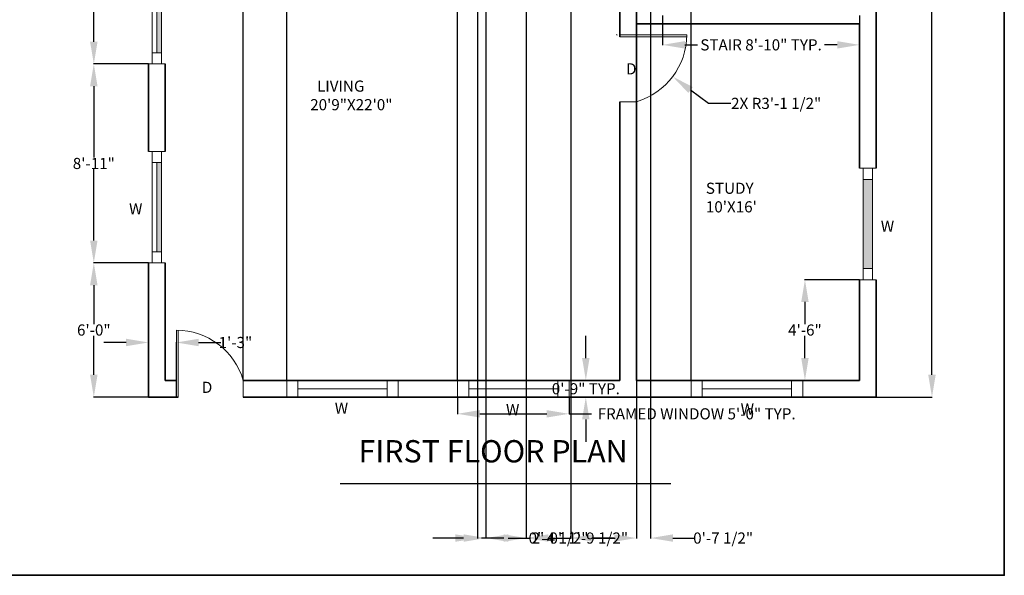
# Model space of a CAD drawing. Units: inches. Extents: x 115 to 1174, y 222 to 1302.
# Tile 3 of 5: x 644 to 1174, y 222 to 521. Entities that reach past the tile are written whole.
import ezdxf

# ---------------------------------------------------------------- set-up
doc = ezdxf.new("R2010")
doc.units = ezdxf.units.IN
doc.header["$MEASUREMENT"] = 0
for name, color, linetype, lineweight in [('A-ANNO-DIMS', 2, 'Continuous', 18), ('A-ANNO-IDEN', 7, 'Continuous', 13), ('A-ANNO-TEXT', 7, 'Continuous', 25), ('A-ANNO-TTLB', 7, 'Continuous', 35), ('A-AREA-IDEN', 7, 'Continuous', 18), ('A-DOOR', 3, 'Continuous', 18), ('A-GLAZ', 4, 'Continuous', 18), ('A-GLAZ-PATT', 8, 'Continuous', 13), ('A-WALL', 7, 'Continuous', 35)]:
    doc.layers.add(name, color=color, linetype=linetype, lineweight=lineweight)
doc.styles.get("Standard").update_dxf_attribs({"font": 'arial.ttf'})
doc.dimstyles.get("Standard").update_dxf_attribs({"dimtxt": 6, "dimasz": 12, "dimexe": 0.18, "dimexo": 0.0625, "dimgap": 0.09, "dimtad": 0, "dimtih": 1, "dimtoh": 1, "dimdec": 1, "dimzin": 0, "dimdsep": 46, "dimlunit": 3, "dimtxsty": 'Standard', "dimcen": 0.09, "dimadec": 0, "dimazin": 0, "dimtfac": 1, "dimtdec": 1, "dimtofl": 0, "dimtmove": 0, "dimatfit": 3, "dimfxl": 1, "dimtolj": 1, "dimtzin": 0, "dimarcsym": 0})

# ---------------------------------------------------------------- blocks, each defined once
blk = doc.blocks.new('*D4')
at = {"layer": 'A-ANNO-DIMS', "color": 0, "lineweight": -2, "transparency": 16777216}
for p, q in [((1105.28, 801.06), (1135.32, 801.06)), ((1135.14, 789.06), (1135.14, 562.72)), ((1135.14, 330.06), (1135.14, 556.41)), ((1105.28, 318.06), (1135.32, 318.06))]:
    blk.add_line(p, q, dxfattribs=at)
at = {"layer": 'A-ANNO-DIMS', "color": 0, "transparency": 16777216}
for points in [[(1133.14, 789.06), (1137.14, 789.06), (1135.14, 801.06)], [(1133.14, 330.06), (1137.14, 330.06), (1135.14, 318.06)]]:
    blk.add_solid(points, dxfattribs=at)
at = {"layer": 'Defpoints', "color": 0, "transparency": 16777216}
for p in [(1105.22, 801.06), (1105.22, 318.06), (1135.14, 318.06)]:
    blk.add_point(p, dxfattribs=at)
at = {"layer": 'A-ANNO-DIMS', "color": 0, "transparency": 16777216, "insert": (1135.14, 559.56), "char_height": 6, "attachment_point": 5}
blk.add_mtext('\\A1;40\'-3.0"', dxfattribs=at)
blk = doc.blocks.new('DOOR-36-SWING')
for p, q in [((0, 0), (0, 36)), ((0, 36), (0, 0)), ((1, 36), (1, 0)), ((36, 0), (36, 9)), ((0, 0), (1, 0))]:
    blk.add_line(p, q)
blk.add_arc((0, -1.5), 37.5, 16.2602, 90)
blk = doc.blocks.new('WIN-60-FULL-FRAME')
for p, q in [((0, 0), (0, 9)), ((0, 9), (60, 9)), ((6, 0), (6, 9)), ((54, 9), (54, 0)), ((60, 9), (60, 0)), ((60, 0), (0, 0)), ((54, 4.5), (6, 4.5))]:
    blk.add_line(p, q)
blk = doc.blocks.new('*D23')
at = {"layer": 'A-ANNO-DIMS', "color": 0, "lineweight": -2, "transparency": 16777216}
for p, q in [((879.96, 318), (879.96, 308.88)), ((939.96, 318), (939.96, 308.88)), ((891.96, 309.06), (927.96, 309.06)), ((939.96, 309.06), (951.96, 309.06))]:
    blk.add_line(p, q, dxfattribs=at)
at = {"layer": 'A-ANNO-DIMS', "color": 0, "transparency": 16777216}
for points in [[(891.96, 311.06), (891.96, 307.06), (879.96, 309.06)], [(927.96, 311.06), (927.96, 307.06), (939.96, 309.06)]]:
    blk.add_solid(points, dxfattribs=at)
at = {"layer": 'Defpoints', "color": 0, "transparency": 16777216}
for p in [(879.96, 318.06), (939.96, 318.06), (939.96, 309.06)]:
    blk.add_point(p, dxfattribs=at)
at = {"layer": 'A-ANNO-DIMS', "color": 0, "transparency": 16777216, "insert": (1008.58, 309.06), "char_height": 6, "attachment_point": 5}
blk.add_mtext('\\A1;FRAMED WINDOW 5\'-0" TYP.', dxfattribs=at)
blk = doc.blocks.new('*D24')
at = {"layer": 'A-ANNO-DIMS', "color": 0, "lineweight": -2, "transparency": 16777216}
for p, q in [((948.96, 339.06), (948.96, 351.06)), ((940.02, 327.06), (949.14, 327.06)), ((940.02, 318.06), (949.14, 318.06)), ((948.96, 306.06), (948.96, 294.06))]:
    blk.add_line(p, q, dxfattribs=at)
at = {"layer": 'A-ANNO-DIMS', "color": 0, "transparency": 16777216}
for points in [[(946.96, 339.06), (950.96, 339.06), (948.96, 327.06)], [(946.96, 306.06), (950.96, 306.06), (948.96, 318.06)]]:
    blk.add_solid(points, dxfattribs=at)
at = {"layer": 'Defpoints', "color": 0, "transparency": 16777216}
for p in [(939.96, 327.06), (948.96, 327.06), (939.96, 318.06)]:
    blk.add_point(p, dxfattribs=at)
at = {"layer": 'A-ANNO-DIMS', "color": 0, "transparency": 16777216, "insert": (948.96, 322.56), "char_height": 6, "attachment_point": 5}
blk.add_mtext('\\A1;0\'-9" TYP.', dxfattribs=at)
blk = doc.blocks.new('*D27')
at = {"layer": 'A-ANNO-DIMS', "color": 0, "lineweight": -2, "transparency": 16777216}
for p, q in [((990.22, 523.5), (990.22, 507.48)), ((1096.22, 523.5), (1096.22, 507.48)), ((1002.22, 507.66), (1009.02, 507.66)), ((1084.22, 507.66), (1077.42, 507.66))]:
    blk.add_line(p, q, dxfattribs=at)
at = {"layer": 'A-ANNO-DIMS', "color": 0, "transparency": 16777216}
for points in [[(1002.22, 509.66), (1002.22, 505.66), (990.22, 507.66)], [(1084.22, 509.66), (1084.22, 505.66), (1096.22, 507.66)]]:
    blk.add_solid(points, dxfattribs=at)
at = {"layer": 'Defpoints', "color": 0, "transparency": 16777216}
for p in [(990.22, 523.56), (1096.22, 523.56), (1096.22, 507.66)]:
    blk.add_point(p, dxfattribs=at)
at = {"layer": 'A-ANNO-DIMS', "color": 0, "transparency": 16777216, "insert": (1043.22, 507.66), "char_height": 6, "attachment_point": 5}
blk.add_mtext('\\A1;STAIR 8\'-10" TYP.', dxfattribs=at)
blk = doc.blocks.new('*D51')
at = {"layer": 'A-ANNO-DIMS', "color": 0, "lineweight": -2, "transparency": 16777216}
for p, q in [((713.66, 390.28), (684.14, 390.28)), ((684.32, 378.28), (684.32, 357.32)), ((684.32, 330.06), (684.32, 351.02)), ((713.66, 318.06), (684.14, 318.06))]:
    blk.add_line(p, q, dxfattribs=at)
at = {"layer": 'A-ANNO-DIMS', "color": 0, "transparency": 16777216}
for points in [[(682.32, 378.28), (686.32, 378.28), (684.32, 390.28)], [(682.32, 330.06), (686.32, 330.06), (684.32, 318.06)]]:
    blk.add_solid(points, dxfattribs=at)
at = {"layer": 'Defpoints', "color": 0, "transparency": 16777216}
for p in [(684.32, 390.28), (713.72, 390.28), (713.72, 318.06)]:
    blk.add_point(p, dxfattribs=at)
at = {"layer": 'A-ANNO-DIMS', "color": 0, "transparency": 16777216, "insert": (684.32, 354.17), "char_height": 6, "attachment_point": 5}
blk.add_mtext('\\A1;6\'-0"', dxfattribs=at)
blk = doc.blocks.new('*D52')
at = {"layer": 'A-ANNO-DIMS', "color": 0, "lineweight": -2, "transparency": 16777216}
for p, q in [((713.66, 497.36), (684.14, 497.36)), ((684.32, 485.36), (684.32, 446.97)), ((684.32, 402.28), (684.32, 440.67)), ((713.66, 390.28), (684.14, 390.28))]:
    blk.add_line(p, q, dxfattribs=at)
at = {"layer": 'A-ANNO-DIMS', "color": 0, "transparency": 16777216}
for points in [[(682.32, 485.36), (686.32, 485.36), (684.32, 497.36)], [(682.32, 402.28), (686.32, 402.28), (684.32, 390.28)]]:
    blk.add_solid(points, dxfattribs=at)
at = {"layer": 'Defpoints', "color": 0, "transparency": 16777216}
for p in [(684.32, 497.36), (713.72, 497.36), (713.72, 390.28)]:
    blk.add_point(p, dxfattribs=at)
at = {"layer": 'A-ANNO-DIMS', "color": 0, "transparency": 16777216, "insert": (684.32, 443.82), "char_height": 6, "attachment_point": 5}
blk.add_mtext('\\A1;8\'-11"', dxfattribs=at)
blk = doc.blocks.new('*D53')
at = {"layer": 'A-ANNO-DIMS', "color": 0, "lineweight": -2, "transparency": 16777216}
for p, q in [((713.66, 641.84), (684.14, 641.84)), ((684.32, 629.84), (684.32, 572.79)), ((684.32, 509.36), (684.32, 566.41)), ((713.66, 497.36), (684.14, 497.36))]:
    blk.add_line(p, q, dxfattribs=at)
at = {"layer": 'A-ANNO-DIMS', "color": 0, "transparency": 16777216}
for points in [[(682.32, 629.84), (686.32, 629.84), (684.32, 641.84)], [(682.32, 509.36), (686.32, 509.36), (684.32, 497.36)]]:
    blk.add_solid(points, dxfattribs=at)
at = {"layer": 'Defpoints', "color": 0, "transparency": 16777216}
for p in [(684.32, 641.84), (713.72, 641.84), (713.72, 497.36)]:
    blk.add_point(p, dxfattribs=at)
at = {"layer": 'A-ANNO-DIMS', "color": 0, "transparency": 16777216, "insert": (684.32, 569.6), "char_height": 6, "attachment_point": 5}
blk.add_mtext('\\A1;12\'-0 1/2"', dxfattribs=at)
blk = doc.blocks.new('*D55')
at = {"layer": 'A-ANNO-DIMS', "color": 0, "lineweight": -2, "transparency": 16777216}
for p, q in [((1096.16, 381.27), (1066.64, 381.27)), ((1066.82, 369.27), (1066.82, 357.32)), ((1066.82, 339.06), (1066.82, 351.02)), ((1096.16, 327.06), (1066.64, 327.06))]:
    blk.add_line(p, q, dxfattribs=at)
at = {"layer": 'A-ANNO-DIMS', "color": 0, "transparency": 16777216}
for points in [[(1064.82, 369.27), (1068.82, 369.27), (1066.82, 381.27)], [(1064.82, 339.06), (1068.82, 339.06), (1066.82, 327.06)]]:
    blk.add_solid(points, dxfattribs=at)
at = {"layer": 'Defpoints', "color": 0, "transparency": 16777216}
for p in [(1066.82, 381.27), (1096.22, 381.27), (1096.22, 327.06)]:
    blk.add_point(p, dxfattribs=at)
at = {"layer": 'A-ANNO-DIMS', "color": 0, "transparency": 16777216, "insert": (1066.82, 354.17), "char_height": 6, "attachment_point": 5}
blk.add_mtext('\\A1;4\'-6"', dxfattribs=at)
blk = doc.blocks.new('*D58')
at = {"layer": 'A-ANNO-DIMS', "color": 0, "lineweight": -2, "transparency": 16777216}
for p, q in [((895.22, 792), (895.22, 242.01)), ((916.83, 792), (916.83, 242.01)), ((883.22, 242.19), (871.22, 242.19)), ((928.83, 242.19), (940.83, 242.19))]:
    blk.add_line(p, q, dxfattribs=at)
at = {"layer": 'A-ANNO-DIMS', "color": 0, "transparency": 16777216}
for points in [[(883.22, 244.19), (883.22, 240.19), (895.22, 242.19)], [(928.83, 244.19), (928.83, 240.19), (916.83, 242.19)]]:
    blk.add_solid(points, dxfattribs=at)
at = {"layer": 'Defpoints', "color": 0, "transparency": 16777216}
for p in [(895.22, 792.06), (916.83, 792.06), (916.83, 242.19)]:
    blk.add_point(p, dxfattribs=at)
at = {"layer": 'A-ANNO-DIMS', "color": 0, "transparency": 16777216, "insert": (955.6, 242.19), "char_height": 6, "attachment_point": 5}
blk.add_mtext('\\A1;1\'-9 1/2"', dxfattribs=at)
blk = doc.blocks.new('*D59')
at = {"layer": 'A-ANNO-DIMS', "color": 0, "lineweight": -2, "transparency": 16777216}
for p, q in [((916.831751, 792.001973), (916.831751, 242.009173)), ((940.831751, 792.001973), (940.831751, 242.009173)), ((904.831751, 242.189173), (892.831751, 242.189173)), ((952.831751, 242.189173), (964.831751, 242.189173))]:
    blk.add_line(p, q, dxfattribs=at)
at = {"layer": 'A-ANNO-DIMS', "color": 0, "transparency": 16777216}
for points in [[(904.831751, 244.189173), (904.831751, 240.189173), (916.831751, 242.189173)], [(952.831751, 244.189173), (952.831751, 240.189173), (940.831751, 242.189173)]]:
    blk.add_solid(points, dxfattribs=at)
at = {"layer": 'Defpoints', "color": 0, "transparency": 16777216}
for p in [(916.831751, 792.064473), (940.831751, 792.064473), (940.831751, 242.189173)]:
    blk.add_point(p, dxfattribs=at)
at = {"layer": 'A-ANNO-DIMS', "color": 0, "transparency": 16777216, "insert": (928.831751, 242.189173), "char_height": 6, "attachment_point": 5}
blk.add_mtext('\\A1;2\'-0"', dxfattribs=at)
blk = doc.blocks.new('*D60')
at = {"layer": 'A-ANNO-DIMS', "color": 0, "lineweight": -2, "transparency": 16777216}
for p, q in [((976.22, 792), (976.22, 242.01)), ((983.78, 792), (983.78, 242.01)), ((964.22, 242.19), (952.22, 242.19)), ((995.78, 242.19), (1007.78, 242.19))]:
    blk.add_line(p, q, dxfattribs=at)
at = {"layer": 'A-ANNO-DIMS', "color": 0, "transparency": 16777216}
for points in [[(964.22, 244.19), (964.22, 240.19), (976.22, 242.19)], [(995.78, 244.19), (995.78, 240.19), (983.78, 242.19)]]:
    blk.add_solid(points, dxfattribs=at)
at = {"layer": 'Defpoints', "color": 0, "transparency": 16777216}
for p in [(976.22, 792.06), (983.78, 792.06), (983.78, 242.19)]:
    blk.add_point(p, dxfattribs=at)
at = {"layer": 'A-ANNO-DIMS', "color": 0, "transparency": 16777216, "insert": (1022.83, 242.19), "char_height": 6, "attachment_point": 5}
blk.add_mtext('\\A1;0\'-7 1/2"', dxfattribs=at)
blk = doc.blocks.new('*D61')
at = {"layer": 'A-ANNO-DIMS', "color": 0, "lineweight": -2, "transparency": 16777216}
for p, q in [((701.72, 347.46), (689.72, 347.46)), ((713.72, 318.13), (713.72, 347.64)), ((728.72, 318.13), (728.72, 347.64)), ((740.72, 347.46), (752.72, 347.46))]:
    blk.add_line(p, q, dxfattribs=at)
at = {"layer": 'A-ANNO-DIMS', "color": 0, "transparency": 16777216}
for points in [[(701.72, 349.46), (701.72, 345.46), (713.72, 347.46)], [(740.72, 349.46), (740.72, 345.46), (728.72, 347.46)]]:
    blk.add_solid(points, dxfattribs=at)
at = {"layer": 'Defpoints', "color": 0, "transparency": 16777216}
for p in [(728.72, 347.46), (713.72, 318.06), (728.72, 318.06)]:
    blk.add_point(p, dxfattribs=at)
at = {"layer": 'A-ANNO-DIMS', "color": 0, "transparency": 16777216, "insert": (760.5, 347.46), "char_height": 6, "attachment_point": 5}
blk.add_mtext('\\A1;1\'-3"', dxfattribs=at)
blk = doc.blocks.new('*D62')
at = {"layer": 'A-ANNO-DIMS', "color": 0, "lineweight": -2, "transparency": 16777216}
for p, q in [((752.72, 830.46), (740.72, 830.46)), ((764.72, 327.13), (764.72, 830.64)), ((788.09, 327.13), (788.09, 830.64)), ((800.09, 830.46), (812.09, 830.46))]:
    blk.add_line(p, q, dxfattribs=at)
at = {"layer": 'A-ANNO-DIMS', "color": 0, "transparency": 16777216}
for points in [[(752.72, 832.46), (752.72, 828.46), (764.72, 830.46)], [(800.09, 832.46), (800.09, 828.46), (788.09, 830.46)]]:
    blk.add_solid(points, dxfattribs=at)
at = {"layer": 'Defpoints', "color": 0, "transparency": 16777216}
for p in [(788.09, 830.46), (764.72, 327.06), (788.09, 327.06)]:
    blk.add_point(p, dxfattribs=at)
at = {"layer": 'A-ANNO-DIMS', "color": 0, "transparency": 16777216, "insert": (829.19, 830.46), "char_height": 6, "attachment_point": 5}
blk.add_mtext('\\A1;1\'-11 1/2"', dxfattribs=at)
blk = doc.blocks.new('*D63')
at = {"layer": 'A-ANNO-DIMS', "color": 0, "lineweight": -2, "transparency": 16777216}
for p, q in [((788.09, 327.13), (788.09, 830.64)), ((800.09, 830.46), (825.98, 830.46)), ((867.96, 830.46), (842.06, 830.46)), ((879.96, 327.13), (879.96, 830.64))]:
    blk.add_line(p, q, dxfattribs=at)
at = {"layer": 'A-ANNO-DIMS', "color": 0, "transparency": 16777216}
for points in [[(800.09, 832.46), (800.09, 828.46), (788.09, 830.46)], [(867.96, 832.46), (867.96, 828.46), (879.96, 830.46)]]:
    blk.add_solid(points, dxfattribs=at)
at = {"layer": 'Defpoints', "color": 0, "transparency": 16777216}
for p in [(879.96, 830.46), (788.09, 327.06), (879.96, 327.06)]:
    blk.add_point(p, dxfattribs=at)
at = {"layer": 'A-ANNO-DIMS', "color": 0, "transparency": 16777216, "insert": (834.02, 830.46), "char_height": 6, "attachment_point": 5}
blk.add_mtext('\\A1;7\'-8"', dxfattribs=at)
blk = doc.blocks.new('*D64')
at = {"layer": 'A-ANNO-DIMS', "color": 0, "lineweight": -2, "transparency": 16777216}
for p, q in [((976.22, 327.13), (976.22, 830.64)), ((988.22, 830.46), (993.61, 830.46)), ((1005.61, 327.13), (1005.61, 830.64)), ((1005.61, 830.46), (1017.61, 830.46))]:
    blk.add_line(p, q, dxfattribs=at)
at = {"layer": 'A-ANNO-DIMS', "color": 0, "transparency": 16777216}
for points in [[(988.22, 832.46), (988.22, 828.46), (976.22, 830.46)], [(993.61, 832.46), (993.61, 828.46), (1005.61, 830.46)]]:
    blk.add_solid(points, dxfattribs=at)
at = {"layer": 'Defpoints', "color": 0, "transparency": 16777216}
for p in [(1005.61, 830.46), (976.22, 327.06), (1005.61, 327.06)]:
    blk.add_point(p, dxfattribs=at)
at = {"layer": 'A-ANNO-DIMS', "color": 0, "transparency": 16777216, "insert": (1032.72, 830.46), "char_height": 6, "attachment_point": 5}
blk.add_mtext('\\A1;2\'-5 1/2"', dxfattribs=at)
blk = doc.blocks.new('*D67')
at = {"layer": 'A-ANNO-DIMS', "color": 0, "lineweight": -2, "transparency": 16777216}
for p, q in [((890.72, 733), (890.72, 242.01)), ((895.22, 727.5), (895.22, 242.01)), ((878.72, 242.19), (866.72, 242.19)), ((907.22, 242.19), (919.22, 242.19))]:
    blk.add_line(p, q, dxfattribs=at)
at = {"layer": 'A-ANNO-DIMS', "color": 0, "transparency": 16777216}
for points in [[(878.72, 244.19), (878.72, 240.19), (890.72, 242.19)], [(907.22, 244.19), (907.22, 240.19), (895.22, 242.19)]]:
    blk.add_solid(points, dxfattribs=at)
at = {"layer": 'Defpoints', "color": 0, "transparency": 16777216}
for p in [(890.72, 733.06), (895.22, 727.56), (895.22, 242.19)]:
    blk.add_point(p, dxfattribs=at)
at = {"layer": 'A-ANNO-DIMS', "color": 0, "transparency": 16777216, "insert": (934.28, 242.19), "char_height": 6, "attachment_point": 5}
blk.add_mtext('\\A1;0\'-4 1/2"', dxfattribs=at)
blk = doc.blocks.new('*D94')
at = {"layer": 'A-ANNO-DIMS', "color": 0, "lineweight": -2, "transparency": 16777216}
for p, q in [((965.63, 513.06), (965.81, 513.06)), ((965.72, 512.97), (965.72, 513.15)), ((1014.92, 476.16), (1005.32, 483.36)), ((1026.92, 476.16), (1014.92, 476.16))]:
    blk.add_line(p, q, dxfattribs=at)
at = {"layer": 'A-ANNO-DIMS', "color": 0, "transparency": 16777216}
blk.add_solid([(1006.52, 484.96), (1004.12, 481.76), (995.72, 490.56)], dxfattribs=at)
at = {"layer": 'Defpoints', "color": 0, "transparency": 16777216}
for p in [(965.72, 513.06), (995.72, 490.56)]:
    blk.add_point(p, dxfattribs=at)
at = {"layer": 'A-ANNO-DIMS', "color": 0, "transparency": 16777216, "insert": (1051.35, 476.16), "char_height": 6, "attachment_point": 5}
blk.add_mtext('\\A1;2X R3\'-1 1/2"', dxfattribs=at)

msp = doc.modelspace()

# ---------------------------------------------------------------- hatches: boundary and pattern name
at = {"layer": 'A-GLAZ-PATT'}
h = msp.add_hatch(color=256, dxfattribs=at)
h.dxf.hatch_style = 1
h.paths.add_polyline_path([(720.72, 695.84), (718.22, 695.84), (718.22, 647.84), (720.72, 647.84)])
h.paths.add_polyline_path([(720.72, 551.36), (718.22, 551.36), (718.22, 503.36), (720.72, 503.36)])
h.paths.add_polyline_path([(720.72, 444.28), (718.22, 444.28), (718.22, 396.28), (720.72, 396.28)])
h = msp.add_hatch(color=256, dxfattribs=at)
h.dxf.hatch_style = 1
h.paths.add_polyline_path([(1103.22, 662.55), (1098.22, 662.55), (1098.22, 614.55), (1103.22, 614.55)])
h.paths.add_polyline_path([(1103.22, 435.27), (1098.22, 435.27), (1098.22, 387.27), (1103.22, 387.27)])

# ---------------------------------------------------------------- linework, layer by layer
at = {"layer": 'A-ANNO-TEXT'}
msp.add_line((816.84, 271.59), (994.75, 271.59), dxfattribs=at)
at = {"layer": 'A-ANNO-TTLB'}
msp.add_lwpolyline([(114.85, 1302.15), (1174.06, 1302.15), (1174.06, 222.13), (114.85, 222.13)], close=True, dxfattribs=at)
at = {"layer": 'A-GLAZ'}
for p, q in [((715.72, 497.36), (715.72, 557.36)), ((720.72, 557.36), (720.72, 497.36)), ((718.22, 551.36), (718.22, 503.36)), ((720.72, 503.36), (715.72, 503.36)), ((722.72, 497.36), (713.72, 497.36)), ((713.72, 450.28), (722.72, 450.28)), ((715.72, 390.28), (715.72, 450.28)), ((720.72, 450.28), (720.72, 390.28)), ((715.72, 444.28), (720.72, 444.28)), ((718.22, 444.28), (718.22, 396.28)), ((1096.22, 441.27), (1105.22, 441.27)), ((1098.22, 381.27), (1098.22, 441.27)), ((1103.22, 441.27), (1103.22, 381.27)), ((1098.22, 435.27), (1103.22, 435.27)), ((720.72, 396.28), (715.72, 396.28)), ((722.72, 390.28), (713.72, 390.28)), ((1103.22, 387.27), (1098.22, 387.27)), ((1105.22, 381.27), (1096.22, 381.27))]:
    msp.add_line(p, q, dxfattribs=at)
at = {"layer": 'A-WALL'}
for p, q in [((1105.22, 608.55), (1105.22, 441.27)), ((967.22, 591.06), (967.22, 512.06)), ((967.22, 519.06), (967.22, 513.06)), ((976.22, 519.06), (1096.22, 519.06)), ((976.22, 519.06), (976.22, 513.06)), ((1096.22, 519.06), (1096.22, 441.27)), ((713.72, 497.36), (713.72, 450.28)), ((722.72, 497.36), (722.72, 450.28)), ((967.22, 477.06), (967.22, 327.06)), ((976.22, 477.06), (976.22, 327.06)), ((713.72, 390.28), (713.72, 318.06)), ((722.72, 390.28), (722.72, 327.06)), ((1096.22, 381.27), (1096.22, 327.06)), ((1105.22, 381.27), (1105.22, 318.06)), ((722.72, 327.06), (728.72, 327.06)), ((764.72, 327.06), (967.22, 327.06)), ((976.22, 327.06), (1096.22, 327.06)), ((713.72, 318.06), (729.72, 318.06)), ((722.72, 318.06), (728.72, 318.06)), ((764.72, 318.06), (1105.22, 318.06))]:
    msp.add_line(p, q, dxfattribs=at)

# ---------------------------------------------------------------- block references
at = {"layer": 'A-DOOR', "rotation": 270.0000000000002}
msp.add_blockref('DOOR-36-SWING', (967.22, 513.06), dxfattribs=at)
at = {"layer": 'A-DOOR'}
msp.add_blockref('DOOR-36-SWING', (728.72, 318.06), dxfattribs=at)
at = {"layer": 'A-GLAZ'}
for p in [(788.09, 318.06), (879.96, 318.06), (1005.61, 318.06)]:
    msp.add_blockref('WIN-60-FULL-FRAME', p, dxfattribs=at)

# ---------------------------------------------------------------- texts
at = {"layer": 'A-ANNO-IDEN', "char_height": 6, "attachment_point": 1}
for s, width, insert in [('D', 9.3758, (970.59, 497.74)), ('W', 10.5593, (703.28, 422.41)), ('W', 10.5593, (1107.62, 413.03)), ('D', 9.3758, (742.44, 326.33)), ('W', 10.5593, (813.92, 315.12)), ('W', 10.5593, (906.03, 314.32)), ('W', 10.5593, (1032.24, 314.63))]:
    msp.add_mtext_dynamic_manual_height_columns(s, width=width, gutter_width=30, heights=[0], dxfattribs=dict(at, insert=insert))
at = {"layer": 'A-ANNO-TEXT', "insert": (826.69, 294.9), "char_height": 12, "attachment_point": 1}
msp.add_mtext_dynamic_manual_height_columns('FIRST FLOOR PLAN', width=181.7331, gutter_width=30, heights=[0], dxfattribs=at)
at = {"layer": 'A-AREA-IDEN', "char_height": 6, "attachment_point": 1}
for s, width, insert in [('  LIVING\\P20\'9"X22\'0"', 88.4292, (800.71, 488.46)), ("STUDY\\P10'X16'", 126.6157, (1013.54, 433.48))]:
    msp.add_mtext_dynamic_manual_height_columns(s, width=width, gutter_width=30, heights=[0], dxfattribs=dict(at, insert=insert))

# ---------------------------------------------------------------- dimensions: what is measured, and where the dimension line sits
at = {"layer": 'A-ANNO-DIMS'}
for base, p1, p2, picture, middle in [((788.09, 830.46), (764.72, 327.06), (788.09, 327.06), '*D62', (829.19, 830.46)), ((1005.61, 830.46), (976.22, 327.06), (1005.61, 327.06), '*D64', (1032.72, 830.46)), ((879.96, 830.46), (788.09, 327.06), (879.96, 327.06), '*D63', (834.02, 830.46)), ((916.83, 242.19), (895.22, 792.06), (916.83, 792.06), '*D58', (955.6, 242.19)), ((940.83, 242.19), (916.83, 792.06), (940.83, 792.06), '*D59', (928.83, 242.19)), ((983.78, 242.19), (976.22, 792.06), (983.78, 792.06), '*D60', (1022.83, 242.19)), ((895.22, 242.19), (890.72, 733.06), (895.22, 727.56), '*D67', (934.28, 242.19)), ((728.72, 347.46), (713.72, 318.06), (728.72, 318.06), '*D61', (760.5, 347.46))]:
    dim = msp.add_linear_dim(base=base, p1=p1, p2=p2, dimstyle='Standard', override={"dimdec": 1, "dimlfac": 1, "dimrnd": 0, "dimzin": 1, "dimdsep": 46, "dimlunit": 4, "dimfrac": 2}, dxfattribs=at)
    dim.commit()
    dim.dimension.update_dxf_attribs({"geometry": picture, "text_midpoint": middle})
for base, p1, p2, override, picture, middle in [((1135.14, 318.06), (1105.22, 801.06), (1105.22, 318.06), {"dimclrd": 0, "dimclre": 0, "dimclrt": 0}, '*D4', (1135.14, 559.56)), ((684.32, 641.84), (713.72, 497.36), (713.72, 641.84), {"dimdec": 1, "dimlfac": 1, "dimrnd": 0, "dimzin": 1, "dimdsep": 46, "dimlunit": 4, "dimfrac": 2}, '*D53', (684.32, 569.6)), ((684.32, 497.36), (713.72, 390.28), (713.72, 497.36), {"dimdec": 1, "dimlfac": 1, "dimrnd": 0, "dimzin": 1, "dimdsep": 46, "dimlunit": 4, "dimfrac": 2}, '*D52', (684.32, 443.82)), ((684.32, 390.28), (713.72, 318.06), (713.72, 390.28), {"dimdec": 1, "dimlfac": 1, "dimrnd": 0, "dimzin": 1, "dimdsep": 46, "dimlunit": 4, "dimfrac": 2}, '*D51', (684.32, 354.17)), ((1066.82, 381.27), (1096.22, 327.06), (1096.22, 381.27), {"dimdec": 1, "dimlfac": 1, "dimrnd": 0, "dimzin": 1, "dimdsep": 46, "dimlunit": 4, "dimfrac": 2}, '*D55', (1066.82, 354.17))]:
    dim = msp.add_linear_dim(base=base, p1=p1, p2=p2, angle=90, dimstyle='Standard', override=override, dxfattribs=at)
    dim.commit()
    dim.dimension.update_dxf_attribs({"geometry": picture, "text_midpoint": middle})
for base, p1, p2, text, picture, middle in [((1096.22, 507.66), (990.22, 523.56), (1096.22, 523.56), 'STAIR <> TYP.', '*D27', (1043.22, 507.66)), ((939.96, 309.06), (879.96, 318.06), (939.96, 318.06), 'FRAMED WINDOW <> TYP.', '*D23', (1008.58, 309.06))]:
    dim = msp.add_linear_dim(base=base, p1=p1, p2=p2, text=text, dimstyle='Standard', override={"dimdec": 1, "dimlfac": 1, "dimrnd": 0, "dimzin": 1, "dimdsep": 46, "dimlunit": 4, "dimfrac": 2}, dxfattribs=at)
    dim.commit()
    dim.dimension.update_dxf_attribs({"geometry": picture, "text_midpoint": middle})
dim = msp.add_radius_dim(center=(965.72, 513.06), mpoint=(995.72, 490.56), text='2X <>', dimstyle='Standard', override={"dimdec": 1, "dimlfac": 1, "dimrnd": 0, "dimzin": 1, "dimdsep": 46, "dimlunit": 4, "dimfrac": 2}, dxfattribs=at)
dim.commit()
dim.dimension.update_dxf_attribs({"geometry": '*D94', "text_midpoint": (1051.35, 476.16)})
dim = msp.add_linear_dim(base=(948.96, 327.06), p1=(939.96, 318.06), p2=(939.96, 327.06), angle=90, text='<> TYP.', dimstyle='Standard', override={"dimdec": 1, "dimlfac": 1, "dimrnd": 0, "dimzin": 1, "dimdsep": 46, "dimlunit": 4, "dimfrac": 2}, dxfattribs=at)
dim.commit()
dim.dimension.update_dxf_attribs({"geometry": '*D24', "text_midpoint": (948.96, 322.56)})

doc.saveas('drawing.dxf')
